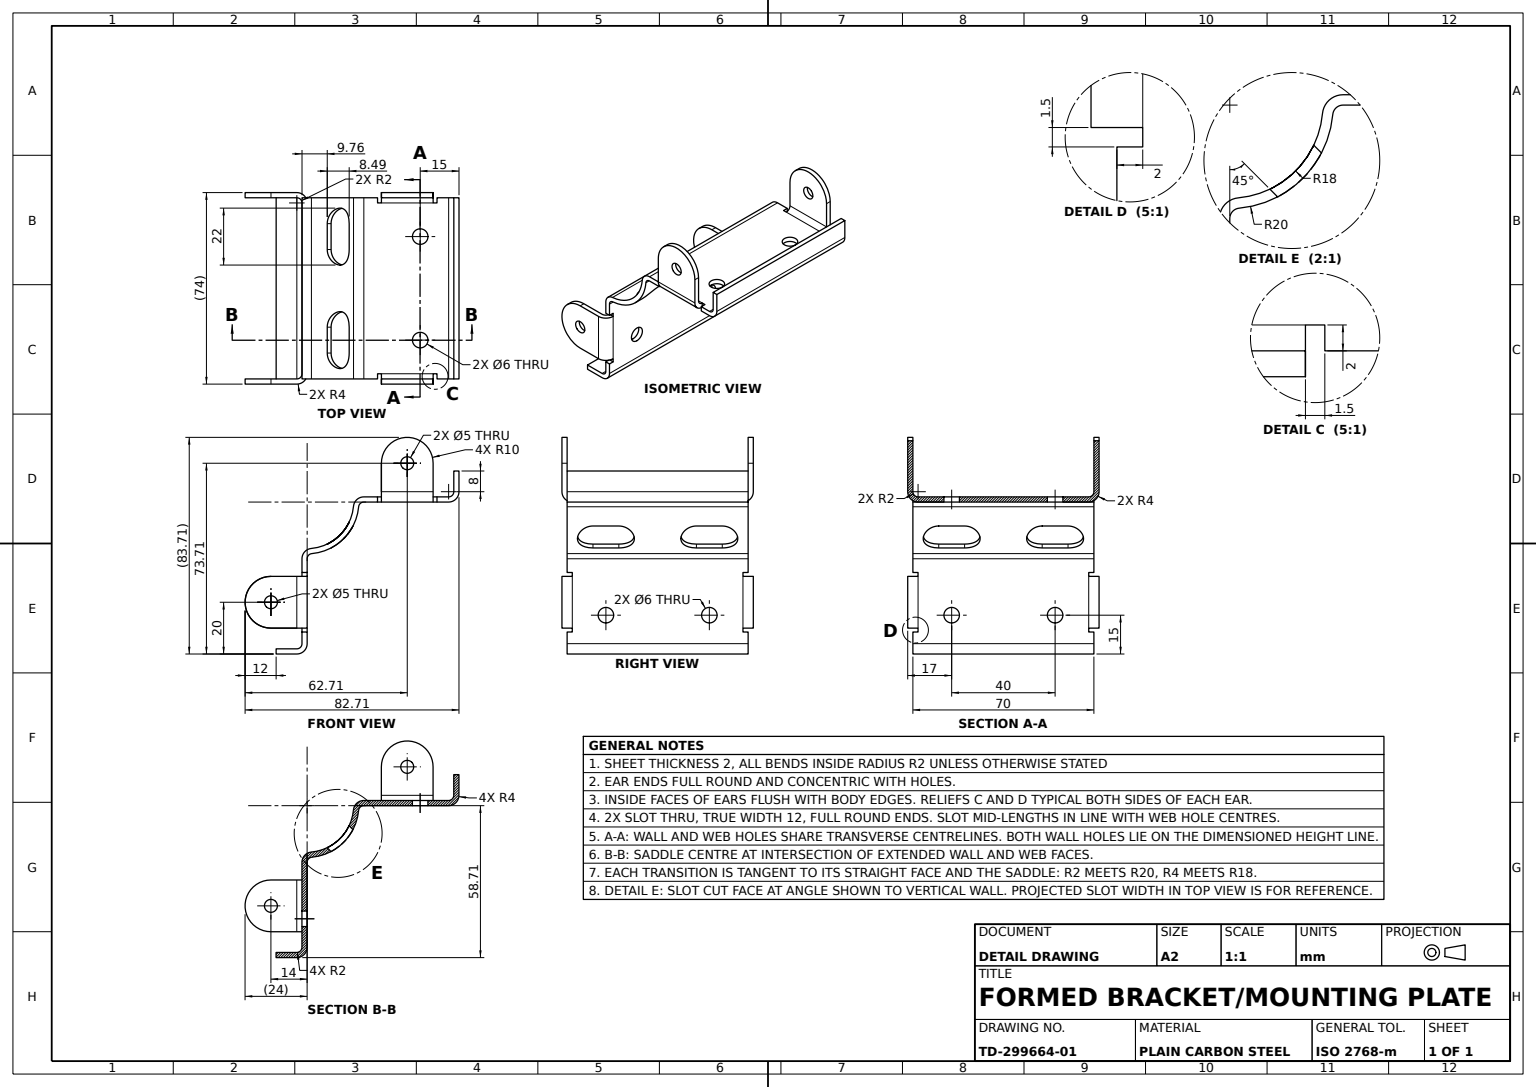
from build123d import *

# Parameters (mm, degrees)
SADDLE_BODY_70MM_DEPTH     = 70
FLANGE_NOTCHES_DEPTH       = 70
FLANGE_HOLES_A_SKETCH_R    = 3.0000000000000018
FLANGE_HOLES_A_SKETCH_R_2  = 3
FLANGE_HOLES_A_6_DEPTH     = 70
FLANGE_HOLES_B_SKETCH_R    = 3.0000000000000018
FLANGE_HOLES_B_6_DEPTH     = 70
SADDLE_SLOT_A_SKETCH_W     = 2
SADDLE_SLOT_A_SKETCH_H     = 1.5
SADDLE_SLOT_A_DEPTH        = 70
SADDLE_SLOT_B_SKETCH_W     = 2
SADDLE_SLOT_B_SKETCH_H     = 1.5
SADDLE_SLOT_B_DEPTH        = 70
MOUNTING_EARS_A_SKETCH_R   = 10.000000000000002
MOUNTING_EARS_A_SKETCH_R_2 = 2.5000000000000027
MOUNTING_EARS_A_SKETCH_R_3 = 9.999999999999508
MOUNTING_EARS_A_DEPTH      = 2
MOUNTING_START             = 2
MOUNTING_EARS_B_SKETCH_R   = 2.5000000000000027
MOUNTING_EARS_B_DEPTH      = 2
EAR_FILLETS_R4_R           = 4
EAR_ROOT_FILLETS_R2_R      = 2


with BuildPart() as part:
    # Saddle Profile Sketch → Saddle Body 70mm (new body)
    with BuildSketch(Plane.XY):
        with BuildLine():
            ThreePointArc((-42.928932188134524, -37.27207793864201), (-41.51471862576144, -37.85786437626892), (-40.100505063388304, -37.27207793864207))
            Line((-40.100505063388304, -37.27207793864207), (-16.906146947202778, -14.077719822456547))
            ThreePointArc((-16.906146947202778, -14.077719822456547), (-14.259726515433778, -12.910289897243185), (-11.518134400191764, -13.832302047711334))
            ThreePointArc((-11.518134400191764, -13.832302047711334), (1.1e-15, -18), (11.51813440019177, -13.832302047711329))
            ThreePointArc((11.51813440019177, -13.832302047711329), (14.259726515433789, -12.910289897243175), (16.90614694720279, -14.077719822456542))
            Line((16.90614694720279, -14.077719822456542), (40.10050506338834, -37.27207793864201))
            ThreePointArc((40.10050506338834, -37.27207793864201), (41.51471862576144, -37.857864376268914), (42.92893218813454, -37.272077938642))
            Line((42.92893218813454, -37.272077938642), (48.585786437626965, -31.615223689149577))
            Line((48.585786437626965, -31.615223689149577), (50.00000000000004, -33.029437251522666))
            Line((50.00000000000004, -33.029437251522666), (44.34314575050763, -38.6862915010151))
            ThreePointArc((44.34314575050763, -38.6862915010151), (41.514718625761446, -39.857864376268886), (38.686291501015276, -38.68629150101508))
            Line((38.686291501015276, -38.68629150101508), (15.491933384829723, -15.491933384829608))
            ThreePointArc((15.491933384829723, -15.491933384829608), (14.168723168945196, -14.908218422222957), (12.797927111324189, -15.369224497457033))
            ThreePointArc((12.797927111324189, -15.369224497457033), (5.67e-15, -20), (-12.797927111324178, -15.36922449745704))
            ThreePointArc((-12.797927111324178, -15.36922449745704), (-14.168723168945185, -14.90821842222296), (-15.491933384829686, -15.491933384829643))
            Line((-15.491933384829686, -15.491933384829643), (-38.68629150101524, -38.68629150101511))
            ThreePointArc((-38.68629150101524, -38.68629150101511), (-41.51471862576143, -39.85786437626892), (-44.343145750507624, -38.686291501015106))
            Line((-44.343145750507624, -38.686291501015106), (-49.999999999999986, -33.02943725152272))
            Line((-49.999999999999986, -33.02943725152272), (-48.58578643762691, -31.61522368914963))
            Line((-48.58578643762691, -31.61522368914963), (-42.928932188134524, -37.27207793864201))
        make_face()
    extrude(amount=SADDLE_BODY_70MM_DEPTH)

    # Flange Notches Sketch → Flange Notches (cut)
    with BuildSketch(Plane(origin=(0, 0, 0), x_dir=(1, 0, 0), z_dir=(0, 1, 0))):
        with BuildLine():
            Line((-6.000000000000002, -10), (-6.000000000000002, -19.999999999999996))
            ThreePointArc((-6.000000000000002, -19.999999999999996), (-1.71e-15, -26), (6, -19.999999999999996))
            Line((6, -19.999999999999996), (6, -10))
            ThreePointArc((6, -10), (-4.3e-16, -3.999999999999999), (-6.000000000000002, -10))
        make_face()
        with BuildLine():
            Line((-6.000000000000001, -50), (-5.999999999999999, -60.00000000000001))
            ThreePointArc((-5.999999999999999, -60.00000000000001), (-1.97e-15, -66), (5.999999999999997, -60.00000000000001))
            Line((5.999999999999997, -60.00000000000001), (5.999999999999999, -50))
            ThreePointArc((5.999999999999999, -50), (-5e-16, -44), (-6.000000000000001, -50))
        make_face()
    extrude(amount=-FLANGE_NOTCHES_DEPTH, mode=Mode.SUBTRACT)

    # Flange Holes A Sketch → Flange Holes A Ø6 (cut)
    with BuildSketch(Plane(origin=(1.4142135623730954, 1.4142135623731005, 0), x_dir=(0, 0, -1), z_dir=(0.7071067811865465, 0.7071067811865487, 0))):
        with Locations(Location((-55.00000000000001, -43.710678118654656, 0), (0, 0, 90))):
            Circle(FLANGE_HOLES_A_SKETCH_R)
        with Locations(Location((-15, -43.710678118654656, 0), (0, 0, 90))):
            Circle(FLANGE_HOLES_A_SKETCH_R_2)
    extrude(amount=-FLANGE_HOLES_A_6_DEPTH, mode=Mode.SUBTRACT)

    # Flange Holes B Sketch → Flange Holes B Ø6 (cut)
    with BuildSketch(Plane(origin=(-1.414213562373113, 1.4142135623731131, 0), x_dir=(0, 0, 1), z_dir=(-0.7071067811865476, 0.7071067811865476, 0))):
        with Locations(Location((15, -43.710678118654634, 0), (0, 0, 270))):
            Circle(FLANGE_HOLES_B_SKETCH_R)
        with Locations(Location((55.00000000000001, -43.710678118654634, 0), (0, 0, 270))):
            Circle(FLANGE_HOLES_B_SKETCH_R)
    extrude(amount=-FLANGE_HOLES_B_6_DEPTH, mode=Mode.SUBTRACT)

    # Saddle Slot A Sketch → Saddle Slot A (cut)
    with BuildSketch(Plane(origin=(-1.414213562373113, 1.4142135623731131, 0), x_dir=(0, 0, 1), z_dir=(-0.7071067811865476, 0.7071067811865476, 0))):
        with Locations((69, -27.96067811865464)):
            Rectangle(SADDLE_SLOT_A_SKETCH_W, SADDLE_SLOT_A_SKETCH_H)
        with Locations((69, -49.460678118654634)):
            Rectangle(SADDLE_SLOT_A_SKETCH_W, SADDLE_SLOT_A_SKETCH_H)
        Polygon((2.000000000000001, -27.210678118654652), (2.000000000000001, -28.710678118654638), (0, -28.710678118654638), (-2.8e-16, -27.210678118654652), align=None)
        Polygon((1.9999999999999913, -48.71067811865465), (1.999999999999994, -50.21067811865465), (2.8e-16, -50.21067811865465), (3.67e-15, -48.71067811865465), align=None)
    extrude(amount=-SADDLE_SLOT_A_DEPTH, mode=Mode.SUBTRACT)

    # Saddle Slot B Sketch → Saddle Slot B (cut)
    with BuildSketch(Plane(origin=(1.4142135623730954, 1.4142135623731005, 0), x_dir=(0, 0, -1), z_dir=(0.7071067811865465, 0.7071067811865487, 0))):
        with Locations((-69, -49.46067811865466)):
            Rectangle(SADDLE_SLOT_B_SKETCH_W, SADDLE_SLOT_B_SKETCH_H)
        with Locations((-69, -27.96067811865466)):
            Rectangle(SADDLE_SLOT_B_SKETCH_W, SADDLE_SLOT_B_SKETCH_H)
        Polygon((-2.000000000000001, -50.210678118654656), (-2.000000000000001, -48.71067811865466), (0, -48.71067811865466), (9e-17, -50.210678118654656), align=None)
        Polygon((-2.0000000000000013, -28.71067811865466), (0, -28.71067811865466), (0, -27.21067811865466), (-2.000000000000001, -27.21067811865466), align=None)
    extrude(amount=-SADDLE_SLOT_B_DEPTH, mode=Mode.SUBTRACT)

    # Mounting Ears A Sketch → Mounting Ears A (add)
    # profile 1 of 5: a face of its own
    with BuildSketch(Plane.XY.offset(70)):
        with Locations((-37.272077938642106, -17.473088065418725)):
            Circle(MOUNTING_EARS_A_SKETCH_R)
        with Locations((-37.272077938642106, -17.473088065418725)):
            Circle(MOUNTING_EARS_A_SKETCH_R_2, mode=Mode.SUBTRACT)
    # profile 2 of 5: a face of its own
    with BuildSketch(Plane.XY.offset(70)):
        with BuildLine():
            Line((-34.44365081389593, -34.44365081389581), (-20.301515190164952, -20.30151519016488))
            Line((-20.301515190164952, -20.30151519016488), (-30.20101012677664, -10.402020253553237))
            ThreePointArc((-30.20101012677664, -10.402020253553237), (-28.033282613529238, -13.646253741767818), (-27.272077938642106, -17.473088065418725))
            ThreePointArc((-27.272077938642106, -17.47308806541873), (-33.445243614991206, -26.711883390531593), (-44.343145750507574, -24.54415587728421))
            Line((-44.34314575050757, -24.544155877284215), (-34.44365081389593, -34.44365081389581))
        make_face()
    # profile 3 of 5: a face of its own
    with BuildSketch(Plane.XY.offset(70)):
        with BuildLine():
            Line((21.715728752538062, -18.887301627791807), (35.85786437626904, -33.02943725152273))
            Line((35.85786437626899, -33.02943725152268), (45.05025253169403, -23.83704909609701))
            ThreePointArc((45.05025253169403, -23.837049096097015), (30.908116907963546, -23.83704909609726), (30.908116907963763, -9.694913472366775))
            Line((30.908116907963763, -9.694913472366776), (21.71572875253811, -18.88730162779185))
        make_face()
    # profile 4 of 5: a face of its own
    with BuildSketch(Plane.XY.offset(70)):
        with Locations((37.979184719828666, -16.765981284232126)):
            Circle(MOUNTING_EARS_A_SKETCH_R_3)
        with Locations((37.979184719828666, -16.765981284232126)):
            Circle(MOUNTING_EARS_A_SKETCH_R_2, mode=Mode.SUBTRACT)
    # profile 5 of 5: a face of its own
    with BuildSketch(Plane.XY.offset(70)):
        Polygon((35.85786437626904, -33.02943725152273), (21.715728752538062, -18.887301627791803), (20.30151519016497, -20.301515190164896), (34.44365081389596, -34.443650813895815), align=None)
    extrude(amount=MOUNTING_EARS_A_DEPTH)

    # Mounting Ears B Sketch → Mounting Ears B (add)
    # profile 1 of 2: a face of its own
    with BuildSketch(Plane(origin=(0, 0, 0), x_dir=(-1, 0, 0), z_dir=(0, 0, -1)).offset(MOUNTING_START)):
        with BuildLine():
            Line((-30.90811690796376, -9.694913472366778), (-20.30151519016498, -20.30151519016489))
            Line((-20.30151519016498, -20.30151519016489), (-34.44365081389596, -34.443650813895815))
            Line((-34.44365081389596, -34.443650813895815), (-45.050252531694035, -23.83704909609701))
            ThreePointArc((-45.050252531694035, -23.83704909609701), (-45.050252531693786, -9.694913472366988), (-30.90811690796376, -9.694913472366778))
        make_face()
        with Locations(Location((-37.979184719828666, -16.765981284232126, 0), (0, 0, 180))):
            Circle(MOUNTING_EARS_B_SKETCH_R, mode=Mode.SUBTRACT)
    # profile 2 of 2: a face of its own
    with BuildSketch(Plane(origin=(0, 0, 0), x_dir=(-1, 0, 0), z_dir=(0, 0, -1)).offset(MOUNTING_START)):
        with BuildLine():
            Line((30.201010126776644, -10.402020253553237), (20.301515190164952, -20.30151519016488))
            Line((20.301515190164952, -20.30151519016488), (34.44365081389595, -34.443650813895815))
            Line((34.44365081389595, -34.443650813895815), (44.34314575050756, -24.54415587728423))
            ThreePointArc((44.34314575050756, -24.54415587728423), (44.3431457505076, -10.402020253553266), (30.201010126776644, -10.402020253553237))
        make_face()
        with Locations(Location((37.272077938642106, -17.473088065418725, 0), (0, 0, 180))):
            Circle(MOUNTING_EARS_B_SKETCH_R, mode=Mode.SUBTRACT)
    extrude(amount=-MOUNTING_EARS_B_DEPTH)

    # Ear Fillets R4
    ear_fillets_r4_edges = [part.edges().sort_by_distance(p)[0] for p in [
        (27.372583002030467, -27.372583002030353, -2),
        (27.372583002030463, -27.372583002030353, 72),
        (-27.37258300203044, -27.372583002030346, 72),
        (-27.372583002030453, -27.372583002030346, -2),
    ]]
    fillet(ear_fillets_r4_edges, radius=EAR_FILLETS_R4_R)

    # Ear Root Fillets R2
    ear_root_fillets_r2_edges = [part.edges().sort_by_distance(p)[0] for p in [
        (28.786796564403556, -25.958369439657268, 70),
        (-28.786796564403513, -25.958369439657282, 70),
        (28.786796564403556, -25.958369439657268, 0),
        (-28.786796564403524, -25.95836943965729, 0),
    ]]
    fillet(ear_root_fillets_r2_edges, radius=EAR_ROOT_FILLETS_R2_R)


solid = part.part
